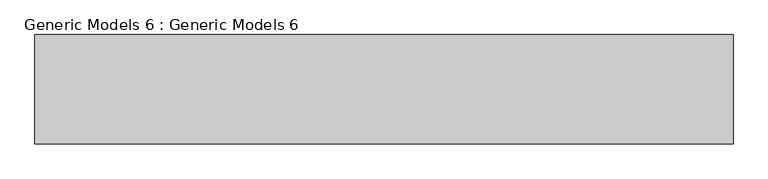
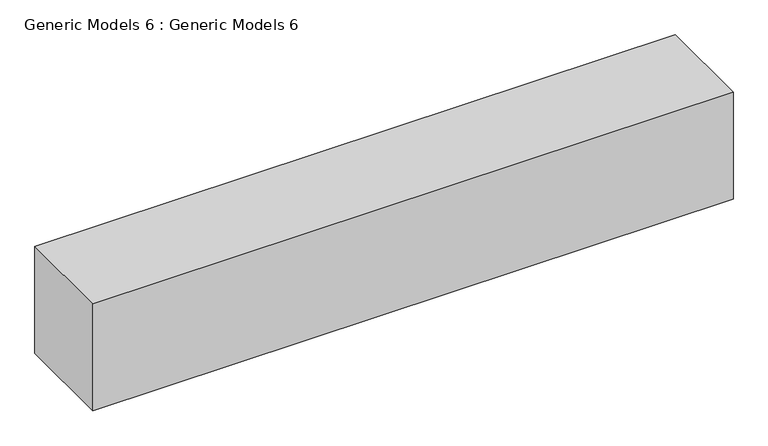
"""IFC4 building model written with IfcOpenShell, lengths in millimetres: proxy geometry, Generic Models 6 : Generic Models 6."""

from ifc_helpers import new_model, si_unit, frame, origin, place, context, project, spatial, polyline, outline, extrude, source, transform, mapped, element, save


def generic_models_6_generic_models_6_32940019(model_context):
    return source(origin(), model_context, "Body", "SweptSolid", [
        extrude(outline(polyline([(-5746.8607439, -6341.8842658), (-9699.7357439, -6341.8842658), (-9699.7357439, -5722.5827462), (-5746.8607439, -5722.5827462), (-5746.8607439, -6341.8842658)])), frame((0.0, 0.0, 3352.8), z_axis=(0.0, 0.0, 1.0), x_axis=(1.0, 0.0, 0.0)), (0.0, 0.0, 1.0), 698.5),
    ])


if __name__ == "__main__":
    model = new_model("IFC4")
    model_context = context("Model", 3, world=origin())
    ifc_project = project(units=[si_unit("LENGTHUNIT", "METRE", prefix="MILLI")], contexts=[model_context])
    site = spatial("IfcSite", under=ifc_project)
    building = spatial("IfcBuilding", under=site)
    placement = place(None, origin())
    generic_models_6_generic_models_6_shape = generic_models_6_generic_models_6_32940019(model_context)
    element("IfcBuildingElementProxy", 1, Name="Generic Models 6 : Generic Models 6", ObjectType="Generic Models 6 : Generic Models 6", at=placement, inside=building, context=model_context, shape_type="MappedRepresentation", body=[
        mapped(generic_models_6_generic_models_6_shape, transform((0.0, 0.0, 0.0), x_axis=(1.0, 0.0, 0.0), y_axis=(0.0, 1.0, 0.0), z_axis=(0.0, 0.0, 1.0))),
    ])
    save(model, "model.ifc")
